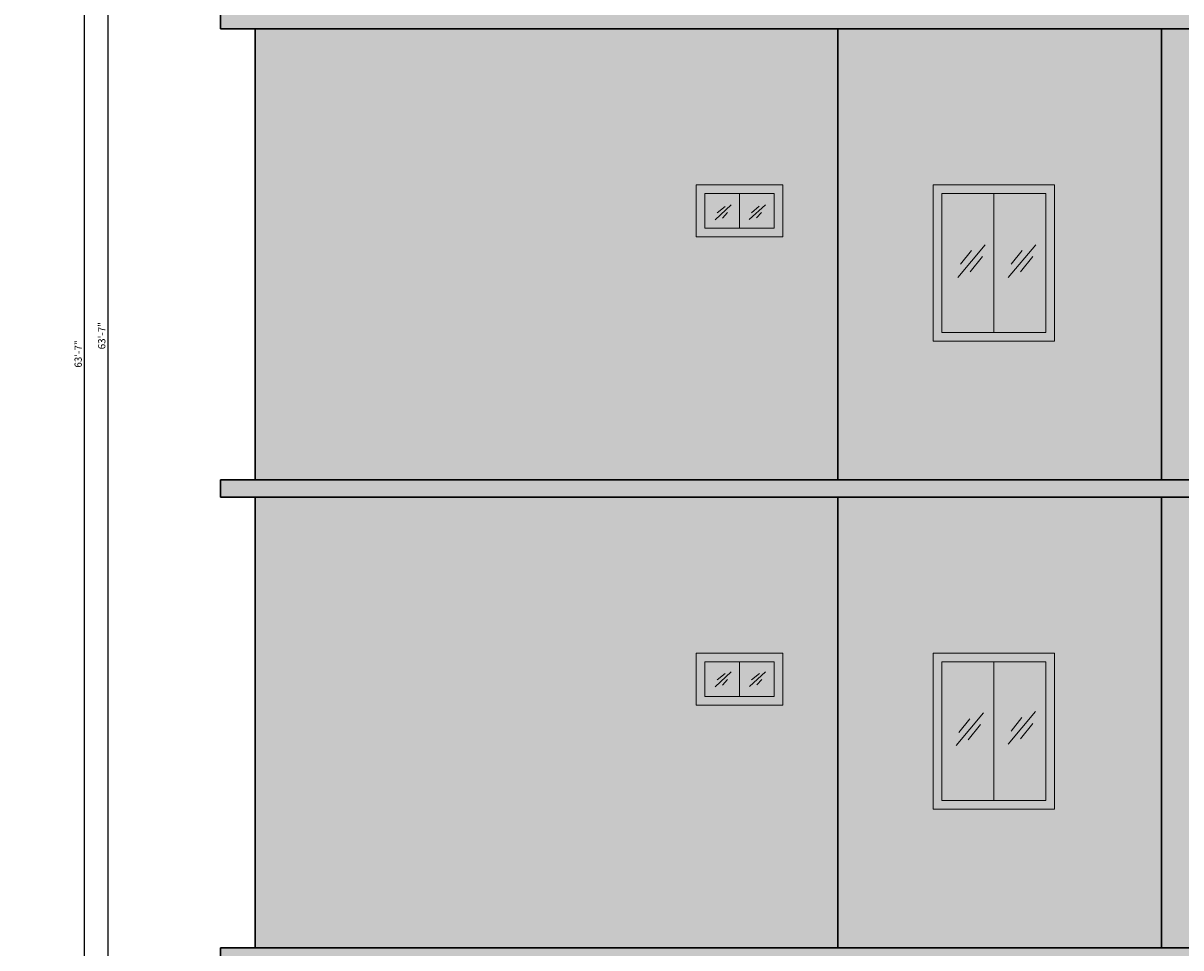
# Model space of a CAD drawing. Units: inches. Extents: x 2391 to 16591, y 7259 to 10239.
# Tile 13 of 27: x 3487 to 3888, y 7746 to 8066. Entities that reach past the tile are written whole.
import ezdxf

# ---------------------------------------------------------------- set-up
doc = ezdxf.new("R2010")
doc.units = ezdxf.units.IN
for name, color, linetype, lineweight in [('A-ANNO-DIMS', 4, 'Continuous', 18), ('A-ELEV', 7, 'Continuous', 30), ('A-ELEV-GLAZ', 4, 'Continuous', 18), ('A-ELEV-GLAZ-PATT', 141, 'Continuous', 13), ('A-ELEV-PATT', 8, 'Continuous', 13), ('A-ELEV-SURF-PATT', 253, 'Continuous', 13)]:
    doc.layers.add(name, color=color, linetype=linetype, lineweight=lineweight)
doc.styles.get("Standard").update_dxf_attribs({"font": 'arial.ttf'})
doc.dimstyles.new('ISO-25', dxfattribs={"dimtxt": 2.5, "dimasz": 2.5, "dimexe": 1.25, "dimexo": 0.625, "dimtad": 1, "dimdec": 0, "dimlunit": 3, "dimtxsty": 'Standard', "dimcen": 2.5, "dimadec": 0, "dimazin": 0, "dimtfac": 1, "dimtdec": 0, "dimtmove": 0, "dimatfit": 3, "dimfxl": 1, "dimarcsym": 0})

# ---------------------------------------------------------------- blocks, each defined once
blk = doc.blocks.new('GLASS-REFLECTION-VENT')
for p, q in [((0, 0), (5.55, 5.12)), ((0.7, 2.37), (3.45, 4.58)), ((2.48, 0.59), (4.26, 2.48))]:
    blk.add_line(p, q)
blk = doc.blocks.new('GLASS-REFLECTION-WINDOW')
for p, q in [((0, 0), (9.5, 11.3)), ((1, 4.52), (4.76, 9.26)), ((4.26, 1.91), (8.52, 7.21))]:
    blk.add_line(p, q)
blk = doc.blocks.new('*D84')
at = {"layer": 'A-ANNO-DIMS', "color": 0, "lineweight": -2, "transparency": 16777216}
for p, q in [((3437.4, 8339.52), (3518.08, 8339.52)), ((3516.83, 7579.02), (3516.83, 8337.02)), ((3464.4, 7576.52), (3518.08, 7576.52))]:
    blk.add_line(p, q, dxfattribs=at)
at = {"layer": 'A-ANNO-DIMS', "color": 0, "transparency": 16777216}
for points in [[(3516.41, 8337.02), (3517.24, 8337.02), (3516.83, 8339.52)], [(3516.41, 7579.02), (3517.24, 7579.02), (3516.83, 7576.52)]]:
    blk.add_solid(points, dxfattribs=at)
at = {"layer": 'Defpoints', "color": 0, "transparency": 16777216}
for p in [(3436.78, 8339.52), (3516.83, 8339.52), (3463.78, 7576.52)]:
    blk.add_point(p, dxfattribs=at)
at = {"layer": 'A-ANNO-DIMS', "color": 0, "transparency": 16777216, "insert": (3514.93, 7958.02), "char_height": 2.5, "attachment_point": 5, "rotation": 90}
blk.add_mtext('63\'-7"', dxfattribs=at)
blk = doc.blocks.new('*D92')
at = {"layer": 'A-ANNO-DIMS', "color": 0, "lineweight": -2, "transparency": 16777216}
for p, q in [((3777.58, 8333.18), (3507.41, 8333.18)), ((3508.66, 7572.68), (3508.66, 8330.68)), ((3561.08, 7570.18), (3507.41, 7570.18))]:
    blk.add_line(p, q, dxfattribs=at)
at = {"layer": 'A-ANNO-DIMS', "color": 0, "transparency": 16777216}
for points in [[(3508.24, 8330.68), (3509.08, 8330.68), (3508.66, 8333.18)], [(3508.24, 7572.68), (3509.08, 7572.68), (3508.66, 7570.18)]]:
    blk.add_solid(points, dxfattribs=at)
at = {"layer": 'Defpoints', "color": 0, "transparency": 16777216}
for p in [(3508.66, 8333.18), (3778.21, 8333.18), (3561.71, 7570.18)]:
    blk.add_point(p, dxfattribs=at)
at = {"layer": 'A-ANNO-DIMS', "color": 0, "transparency": 16777216, "insert": (3506.76, 7951.68), "char_height": 2.5, "attachment_point": 5, "rotation": 90}
blk.add_mtext('63\'-7"', dxfattribs=at)

msp = doc.modelspace()

# ---------------------------------------------------------------- hatches: boundary and pattern name
at = {"layer": 'A-ELEV-GLAZ-PATT'}
h = msp.add_hatch(color=256, dxfattribs=at)
h.dxf.hatch_style = 1
h.paths.add_polyline_path([(3750.21, 8172.18), (3720.21, 8172.18), (3720.21, 8154.18), (3750.21, 8154.18)])
h.paths.add_polyline_path([(3747.21, 8169.18), (3747.21, 8157.18), (3723.21, 8157.18), (3723.21, 8169.18)], flags=16)
h.paths.add_polyline_path([(3802.21, 8172.18), (3802.21, 8118.18), (3844.21, 8118.18), (3844.21, 8172.18)])
h.paths.add_polyline_path([(3841.21, 8169.18), (3841.21, 8121.18), (3805.21, 8121.18), (3805.21, 8169.18)], flags=16)
h.paths.add_polyline_path([(3956.96, 8172.18), (3914.96, 8172.18), (3914.96, 8118.18), (3956.96, 8118.18)])
h.paths.add_polyline_path([(3953.96, 8169.18), (3953.96, 8121.18), (3917.96, 8121.18), (3917.96, 8169.18)], flags=16)
h.paths.add_polyline_path([(3720.21, 8010.18), (3720.21, 7992.18), (3750.21, 7992.18), (3750.21, 8010.18)])
h.paths.add_polyline_path([(3747.21, 8007.18), (3747.21, 7995.18), (3723.21, 7995.18), (3723.21, 8007.18)], flags=16)
h.paths.add_polyline_path([(3802.21, 8010.18), (3802.21, 7956.18), (3844.21, 7956.18), (3844.21, 8010.18)])
h.paths.add_polyline_path([(3841.21, 8007.18), (3841.21, 7959.18), (3805.21, 7959.18), (3805.21, 8007.18)], flags=16)
h.paths.add_polyline_path([(3914.96, 8010.18), (3914.96, 7956.18), (3956.96, 7956.18), (3956.96, 8010.18)])
h.paths.add_polyline_path([(3917.96, 8007.18), (3953.96, 8007.18), (3953.96, 7959.18), (3917.96, 7959.18)], flags=16)
h.paths.add_polyline_path([(3750.21, 7848.18), (3720.21, 7848.18), (3720.21, 7830.18), (3750.21, 7830.18)])
h.paths.add_polyline_path([(3747.21, 7845.18), (3747.21, 7833.18), (3723.21, 7833.18), (3723.21, 7845.18)], flags=16)
h.paths.add_polyline_path([(3844.21, 7848.18), (3802.21, 7848.18), (3802.21, 7794.18), (3844.21, 7794.18)])
h.paths.add_polyline_path([(3805.21, 7845.18), (3841.21, 7845.18), (3841.21, 7797.18), (3805.21, 7797.18)], flags=16)
h.paths.add_polyline_path([(3914.96, 7848.18), (3914.96, 7794.18), (3956.96, 7794.18), (3956.96, 7848.18)])
h.paths.add_polyline_path([(3917.96, 7845.18), (3953.96, 7845.18), (3953.96, 7797.18), (3917.96, 7797.18)], flags=16)
h = msp.add_hatch(color=256, dxfattribs=at)
h.dxf.hatch_style = 1
h.paths.add_polyline_path([(3735.21, 8169.18), (3723.21, 8169.18), (3723.21, 8157.18), (3735.21, 8157.18)])
h.paths.add_polyline_path([(3747.21, 8169.18), (3735.21, 8169.18), (3735.21, 8157.18), (3747.21, 8157.18)])
h.paths.add_polyline_path([(3823.21, 8169.18), (3805.21, 8169.18), (3805.21, 8121.18), (3823.21, 8121.18)])
h.paths.add_polyline_path([(3841.21, 8169.18), (3823.21, 8169.18), (3823.21, 8121.18), (3841.21, 8121.18)])
h.paths.add_polyline_path([(3935.96, 8169.18), (3917.96, 8169.18), (3917.96, 8121.18), (3935.96, 8121.18)])
h.paths.add_polyline_path([(3953.96, 8169.18), (3935.96, 8169.18), (3935.96, 8121.18), (3953.96, 8121.18)])
h.paths.add_polyline_path([(3735.21, 8007.18), (3723.21, 8007.18), (3723.21, 7995.18), (3735.21, 7995.18)])
h.paths.add_polyline_path([(3747.21, 8007.18), (3735.21, 8007.18), (3735.21, 7995.18), (3747.21, 7995.18)])
h.paths.add_polyline_path([(3823.21, 8007.18), (3805.21, 8007.18), (3805.21, 7959.18), (3823.21, 7959.18)])
h.paths.add_polyline_path([(3841.21, 8007.18), (3823.21, 8007.18), (3823.21, 7959.18), (3841.21, 7959.18)])
h.paths.add_polyline_path([(3935.96, 8007.18), (3917.96, 8007.18), (3917.96, 7959.18), (3935.96, 7959.18)])
h.paths.add_polyline_path([(3953.96, 8007.18), (3935.96, 8007.18), (3935.96, 7959.18), (3953.96, 7959.18)])
h.paths.add_polyline_path([(3735.21, 7845.18), (3723.21, 7845.18), (3723.21, 7833.18), (3735.21, 7833.18)])
h.paths.add_polyline_path([(3747.21, 7845.18), (3735.21, 7845.18), (3735.21, 7833.18), (3747.21, 7833.18)])
h.paths.add_polyline_path([(3823.21, 7845.18), (3805.21, 7845.18), (3805.21, 7797.18), (3823.21, 7797.18)])
h.paths.add_polyline_path([(3841.21, 7845.18), (3823.21, 7845.18), (3823.21, 7797.18), (3841.21, 7797.18)])
h.paths.add_polyline_path([(3935.96, 7845.18), (3917.96, 7845.18), (3917.96, 7797.18), (3935.96, 7797.18)])
h.paths.add_polyline_path([(3953.96, 7845.18), (3935.96, 7845.18), (3935.96, 7797.18), (3953.96, 7797.18)])
at = {"layer": 'A-ELEV-PATT'}
h = msp.add_hatch(dxfattribs=at)
h.set_pattern_fill('BRSTONE', color=256)
h.paths.add_polyline_path([(3999.71, 8226.18), (3881.21, 8226.18), (3881.21, 8070.18), (3999.71, 8070.18)])
h.paths.add_polyline_path([(3956.96, 8118.18), (3914.96, 8118.18), (3914.96, 8172.18), (3956.96, 8172.18)], flags=16)
h.paths.add_polyline_path([(3953.96, 8121.18), (3917.96, 8121.18), (3917.96, 8169.18), (3953.96, 8169.18)], flags=0)
h.paths.add_polyline_path([(3999.71, 8064.18), (3881.21, 8064.18), (3881.21, 7908.18), (3999.71, 7908.18)])
h.paths.add_polyline_path([(3956.96, 7956.18), (3914.96, 7956.18), (3914.96, 8010.18), (3956.96, 8010.18)], flags=16)
h.paths.add_polyline_path([(3953.96, 7959.18), (3917.96, 7959.18), (3917.96, 8007.18), (3953.96, 8007.18)], flags=0)
h.paths.add_polyline_path([(3999.71, 7902.18), (3881.21, 7902.18), (3881.21, 7746.18), (3999.71, 7746.18)])
h.paths.add_polyline_path([(3956.96, 7794.18), (3914.96, 7794.18), (3914.96, 7848.18), (3956.96, 7848.18)], flags=16)
h.paths.add_polyline_path([(3953.96, 7797.18), (3917.96, 7797.18), (3917.96, 7845.18), (3953.96, 7845.18)], flags=0)
h.paths.add_polyline_path([(3999.71, 7740.18), (3567.71, 7740.18), (3567.71, 7697.18), (3760.71, 7697.18), (3760.71, 7706.18), (3755.71, 7706.18), (3755.71, 7711.18), (3774.71, 7711.18), (3774.71, 7706.18), (3769.71, 7706.18), (3769.71, 7677.02), (3772.21, 7677.02), (3772.21, 7679.02), (3774.71, 7679.02), (3774.71, 7704.18), (3843.71, 7704.18), (3843.71, 7589.18), (3774.71, 7589.18), (3774.71, 7584.18), (3913.71, 7584.18), (3913.71, 7589.18), (3844.71, 7589.18), (3844.71, 7704.18), (3913.71, 7704.18), (3913.71, 7679.02), (3916.21, 7679.02), (3916.21, 7677.02), (3918.71, 7677.02), (3918.71, 7706.18), (3913.71, 7706.18), (3913.71, 7711.18), (3932.71, 7711.18), (3932.71, 7706.18), (3927.71, 7706.18), (3927.71, 7697.18), (3999.71, 7697.18)])
h.paths.add_polyline_path([(3918.71, 7675.02), (3916.21, 7675.02), (3916.21, 7673.02), (3913.71, 7673.02), (3913.71, 7618.89), (3916.21, 7618.89), (3916.21, 7616.89), (3918.71, 7616.89)], flags=17)
h.paths.add_polyline_path([(3918.71, 7614.89), (3916.21, 7614.89), (3916.21, 7612.89), (3913.71, 7612.89), (3913.71, 7584.18), (3918.71, 7584.18)], flags=17)
h.paths.add_polyline_path([(3774.71, 7673.02), (3772.21, 7673.02), (3772.21, 7675.02), (3769.71, 7675.02), (3769.71, 7616.89), (3772.21, 7616.89), (3772.21, 7618.89), (3774.71, 7618.89)], flags=17)
h.paths.add_polyline_path([(3774.71, 7612.89), (3772.21, 7612.89), (3772.21, 7614.89), (3769.71, 7614.89), (3769.71, 7584.18), (3774.71, 7584.18), (3774.71, 7589.18)], flags=17)
h = msp.add_hatch(dxfattribs=at)
h.set_pattern_fill('GRAVEL', color=256)
h.paths.add_polyline_path([(3769.21, 8226.18), (3567.71, 8226.18), (3567.71, 8070.18), (3769.21, 8070.18)])
h.paths.add_polyline_path([(3720.21, 8154.18), (3720.21, 8172.18), (3750.21, 8172.18), (3750.21, 8154.18)], flags=16)
h.paths.add_polyline_path([(3723.21, 8157.18), (3723.21, 8169.18), (3747.21, 8169.18), (3747.21, 8157.18)], flags=0)
h.paths.add_polyline_path([(3769.21, 8064.18), (3567.71, 8064.18), (3567.71, 7908.18), (3769.21, 7908.18)])
h.paths.add_polyline_path([(3720.21, 7992.18), (3720.21, 8010.18), (3750.21, 8010.18), (3750.21, 7992.18)], flags=16)
h.paths.add_polyline_path([(3723.21, 7995.18), (3723.21, 8007.18), (3747.21, 8007.18), (3747.21, 7995.18)], flags=0)
h.paths.add_polyline_path([(3769.21, 7902.18), (3567.71, 7902.18), (3567.71, 7746.18), (3769.21, 7746.18)])
h.paths.add_polyline_path([(3720.21, 7848.18), (3750.21, 7848.18), (3750.21, 7830.18), (3720.21, 7830.18)], flags=16)
h.paths.add_polyline_path([(3723.21, 7845.18), (3747.21, 7845.18), (3747.21, 7833.18), (3723.21, 7833.18)], flags=0)
h = msp.add_hatch(dxfattribs=at)
h.set_pattern_fill('HONEY', color=256)
h.paths.add_polyline_path([(3881.21, 8226.18), (3769.21, 8226.18), (3769.21, 8070.18), (3881.21, 8070.18)])
h.paths.add_polyline_path([(3844.21, 8118.18), (3802.21, 8118.18), (3802.21, 8172.18), (3844.21, 8172.18)], flags=16)
h.paths.add_polyline_path([(3841.21, 8121.18), (3805.21, 8121.18), (3805.21, 8169.18), (3841.21, 8169.18)], flags=0)
h.paths.add_polyline_path([(3881.21, 8064.18), (3769.21, 8064.18), (3769.21, 7908.18), (3881.21, 7908.18)])
h.paths.add_polyline_path([(3844.21, 7956.18), (3802.21, 7956.18), (3802.21, 8010.18), (3844.21, 8010.18)], flags=16)
h.paths.add_polyline_path([(3841.21, 7959.18), (3805.21, 7959.18), (3805.21, 8007.18), (3841.21, 8007.18)], flags=0)
h.paths.add_polyline_path([(3881.21, 7902.18), (3769.21, 7902.18), (3769.21, 7746.18), (3881.21, 7746.18)])
h.paths.add_polyline_path([(3844.21, 7794.18), (3802.21, 7794.18), (3802.21, 7848.18), (3844.21, 7848.18)], flags=16)
h.paths.add_polyline_path([(3841.21, 7797.18), (3805.21, 7797.18), (3805.21, 7845.18), (3841.21, 7845.18)], flags=0)
at = {"layer": 'A-ELEV-SURF-PATT'}
h = msp.add_hatch(color=256, dxfattribs=at)
h.dxf.hatch_style = 1
h.paths.add_polyline_path([(4011.71, 7740.18), (4011.71, 7746.18), (3555.71, 7746.18), (3555.71, 7740.18)])
h.paths.add_polyline_path([(4011.71, 7902.18), (4011.71, 7908.18), (3555.71, 7908.18), (3555.71, 7902.18)])
h.paths.add_polyline_path([(4011.71, 8064.18), (4011.71, 8070.18), (3555.71, 8070.18), (3555.71, 8064.18)])
h.paths.add_polyline_path([(3555.71, 8232.18), (3555.71, 8226.18), (4011.71, 8226.18), (4011.71, 8232.18)])
h.paths.add_polyline_path([(3778.21, 8333.18), (3778.21, 8328.18), (3978.71, 8328.18), (3978.71, 8333.18)])

# ---------------------------------------------------------------- linework, layer by layer
at = {"layer": 'A-ELEV'}
for p, q in [((3555.71, 8064.18), (3555.71, 8070.18)), ((3555.71, 8064.18), (4011.71, 8064.18)), ((3567.71, 7908.18), (3567.71, 8064.18)), ((3769.21, 8064.18), (3769.21, 7908.18)), ((3881.21, 8064.18), (3881.21, 7908.18)), ((3555.71, 7902.18), (3555.71, 7908.18)), ((3555.71, 7908.18), (4011.71, 7908.18)), ((3555.71, 7902.18), (4011.71, 7902.18)), ((3567.71, 7746.18), (3567.71, 7902.18)), ((3769.21, 7902.18), (3769.21, 7746.18)), ((3881.21, 7902.18), (3881.21, 7746.18)), ((3555.71, 7740.18), (3555.71, 7746.18)), ((3555.71, 7746.18), (4011.71, 7746.18))]:
    msp.add_line(p, q, dxfattribs=at)
at = {"layer": 'A-ELEV-GLAZ'}
for p, q in [((3720.21, 8010.18), (3750.21, 8010.18)), ((3720.21, 8010.18), (3720.21, 7992.18)), ((3750.21, 8010.18), (3750.21, 7992.18)), ((3802.21, 8010.18), (3844.21, 8010.18)), ((3802.21, 7956.18), (3802.21, 8010.18)), ((3844.21, 7956.18), (3844.21, 8010.18)), ((3723.21, 8007.18), (3747.21, 8007.18)), ((3723.21, 8007.18), (3723.21, 7995.18)), ((3735.21, 8007.18), (3735.21, 7995.18)), ((3747.21, 8007.18), (3747.21, 7995.18)), ((3805.21, 8007.18), (3841.21, 8007.18)), ((3805.21, 7959.18), (3805.21, 8007.18)), ((3823.21, 8007.18), (3823.21, 7959.18)), ((3841.21, 7959.18), (3841.21, 8007.18)), ((3723.21, 7995.18), (3747.21, 7995.18)), ((3720.21, 7992.18), (3750.21, 7992.18)), ((3805.21, 7959.18), (3841.21, 7959.18)), ((3802.21, 7956.18), (3844.21, 7956.18)), ((3720.21, 7848.18), (3750.21, 7848.18)), ((3720.21, 7848.18), (3720.21, 7830.18)), ((3750.21, 7848.18), (3750.21, 7830.18)), ((3802.21, 7848.18), (3844.21, 7848.18)), ((3802.21, 7794.18), (3802.21, 7848.18)), ((3844.21, 7794.18), (3844.21, 7848.18)), ((3723.21, 7845.18), (3747.21, 7845.18)), ((3723.21, 7845.18), (3723.21, 7833.18)), ((3735.21, 7845.18), (3735.21, 7833.18)), ((3747.21, 7845.18), (3747.21, 7833.18)), ((3805.21, 7845.18), (3841.21, 7845.18)), ((3805.21, 7797.18), (3805.21, 7845.18)), ((3823.21, 7845.18), (3823.21, 7797.18)), ((3841.21, 7797.18), (3841.21, 7845.18)), ((3720.21, 7830.18), (3750.21, 7830.18)), ((3723.21, 7833.18), (3747.21, 7833.18)), ((3805.21, 7797.18), (3841.21, 7797.18)), ((3802.21, 7794.18), (3844.21, 7794.18))]:
    msp.add_line(p, q, dxfattribs=at)

# ---------------------------------------------------------------- block references
for name, p in [('GLASS-REFLECTION-VENT', (3726.83, 7998.15)), ('GLASS-REFLECTION-VENT', (3738.6, 7998.22)), ('GLASS-REFLECTION-WINDOW', (3810.71, 7978.21)), ('GLASS-REFLECTION-WINDOW', (3828.18, 7978.21)), ('GLASS-REFLECTION-VENT', (3726.83, 7836.53)), ('GLASS-REFLECTION-VENT', (3738.68, 7836.59)), ('GLASS-REFLECTION-WINDOW', (3810.1, 7816.23)), ('GLASS-REFLECTION-WINDOW', (3828.13, 7816.65))]:
    msp.add_blockref(name, p, dxfattribs=at)

# ---------------------------------------------------------------- dimensions: what is measured, and where the dimension line sits
at = {"layer": 'A-ANNO-DIMS'}
for base, p1, p2, picture, middle in [((3516.83, 8339.52), (3463.78, 7576.52), (3436.78, 8339.52), '*D84', (3514.93, 7958.02)), ((3508.66, 8333.18), (3561.71, 7570.18), (3778.21, 8333.18), '*D92', (3506.76, 7951.68))]:
    dim = msp.add_linear_dim(base=base, p1=p1, p2=p2, angle=90, dimstyle='ISO-25', override={"dimdec": 1, "dimlfac": 1, "dimrnd": 0, "dimzin": 1, "dimdsep": 46, "dimlunit": 4, "dimfrac": 2}, dxfattribs=at)
    dim.commit()
    dim.dimension.update_dxf_attribs({"geometry": picture, "text_midpoint": middle})

doc.saveas('drawing.dxf')
